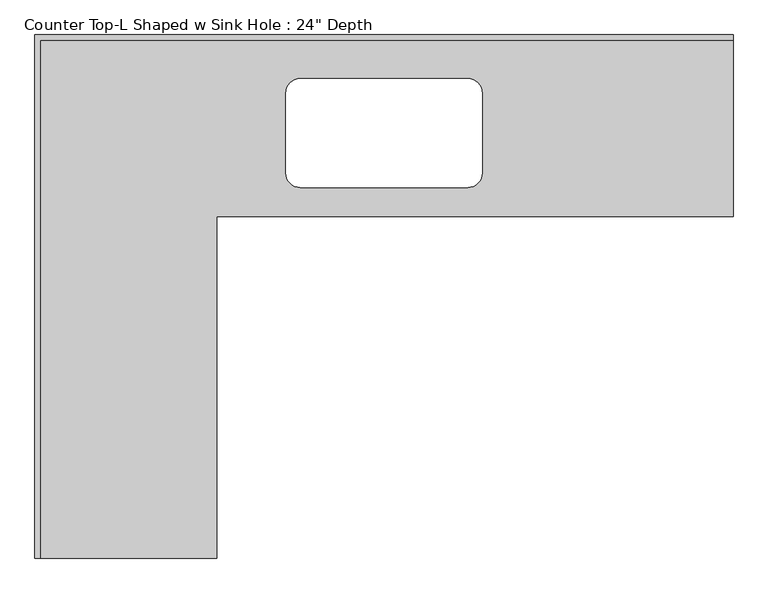
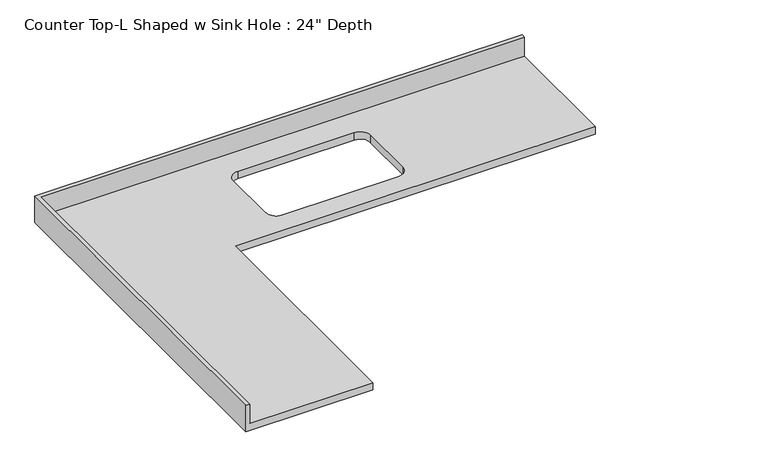
"""IFC4 building model written with IfcOpenShell, lengths in millimetres: furniture geometry."""

from ifc_helpers import new_model, si_unit, frame, origin, place, context, project, spatial, polyline, circle_curve, source, transform, mapped, element, save
from ifc_brep_helpers import plane_surface, revolved_surface, advanced_brep


def furniture_eb5480b5(model_context):
    return source(origin(), model_context, "Body", "AdvancedBrep", [
        advanced_brep(
        [(-565.4622951, -1828.8, 914.4), (-565.4622951, -635.0, 914.4), (1237.9377049, -635.0, 914.4), (1237.9377049, -19.05, 914.4), (-1181.4122951, -19.05, 914.4), (-1181.4122951, -1828.8, 914.4), (310.8377049, -152.4, 914.4), (361.6377049, -203.2, 914.4), (361.6377049, -482.6, 914.4), (310.8377049, -533.4, 914.4), (-273.3622951, -533.4, 914.4), (-324.1622951, -482.6, 914.4), (-324.1622951, -203.2, 914.4), (-273.3622951, -152.4, 914.4), (1237.9377049, 0.0, 876.3), (1237.9377049, -635.0, 876.3), (-565.4622951, -635.0, 876.3), (-565.4622951, -1828.8, 876.3), (-1200.4622951, -1828.8, 876.3), (-1200.4622951, 0.0, 876.3), (310.8377049, -152.4, 876.3), (-273.3622951, -152.4, 876.3), (-324.1622951, -203.2, 876.3), (-324.1622951, -482.6, 876.3), (-273.3622951, -533.4, 876.3), (310.8377049, -533.4, 876.3), (361.6377049, -482.6, 876.3), (361.6377049, -203.2, 876.3), (-1200.4622951, 0.0, 1016.0), (1237.9377049, 0.0, 1016.0), (-1200.4622951, -1828.8, 1016.0), (-1181.4122951, -1828.8, 1016.0), (1237.9377049, -19.05, 1016.0), (-1181.4122951, -19.05, 1016.0)],
        [
            (0, 1),
            (1, 2),
            (2, 3),
            (3, 4),
            (4, 5),
            (5, 0),
            (6, 7, circle_curve(frame((310.8377049, -203.2, 914.4), z_axis=(0.0, 0.0, -1.0), x_axis=(1.0, 0.0, 0.0)), 50.8)),
            (7, 8),
            (8, 9, circle_curve(frame((310.8377049, -482.6, 914.4), z_axis=(0.0, 0.0, -1.0), x_axis=(1.0, 0.0, 0.0)), 50.8)),
            (9, 10),
            (10, 11, circle_curve(frame((-273.3622951, -482.6, 914.4), z_axis=(0.0, 0.0, -1.0), x_axis=(1.0, 0.0, 0.0)), 50.8)),
            (11, 12),
            (12, 13, circle_curve(frame((-273.3622951, -203.2, 914.4), z_axis=(0.0, 0.0, -1.0), x_axis=(1.0, 0.0, 0.0)), 50.8)),
            (13, 6),
            (14, 15),
            (15, 16),
            (16, 17),
            (17, 18),
            (18, 19),
            (19, 14),
            (20, 21),
            (21, 22, circle_curve(frame((-273.3622951, -203.2, 876.3), z_axis=(0.0, 0.0, 1.0), x_axis=(1.0, 0.0, 0.0)), 50.8)),
            (22, 23),
            (23, 24, circle_curve(frame((-273.3622951, -482.6, 876.3), z_axis=(0.0, 0.0, 1.0), x_axis=(1.0, 0.0, 0.0)), 50.8)),
            (24, 25),
            (25, 26, circle_curve(frame((310.8377049, -482.6, 876.3), z_axis=(0.0, 0.0, 1.0), x_axis=(1.0, 0.0, 0.0)), 50.8)),
            (26, 27),
            (27, 20, circle_curve(frame((310.8377049, -203.2, 876.3), z_axis=(0.0, 0.0, 1.0), x_axis=(1.0, 0.0, 0.0)), 50.8)),
            (19, 28),
            (28, 29),
            (29, 14),
            (18, 30),
            (30, 28),
            (17, 0),
            (5, 31),
            (31, 30),
            (16, 1),
            (15, 2),
            (29, 32),
            (32, 3),
            (6, 20),
            (27, 7),
            (26, 8),
            (25, 9),
            (24, 10),
            (23, 11),
            (22, 12),
            (21, 13),
            (31, 33),
            (33, 32),
            (33, 4),
        ],
        [
            plane_surface(frame((-1200.4622951, 0.0, 914.4), z_axis=(0.0, 0.0, 1.0), x_axis=(-1.0, 0.0, 0.0))),
            plane_surface(frame((-1200.4622951, 0.0, 876.3), z_axis=(0.0, 0.0, -1.0), x_axis=(1.0, 0.0, 0.0))),
            plane_surface(frame((1237.9377049, 0.0, 914.4), z_axis=(0.0, 1.0, 0.0), x_axis=(0.0, 0.0, -1.0))),
            plane_surface(frame((-1200.4622951, 0.0, 914.4), z_axis=(-1.0, 0.0, 0.0), x_axis=(0.0, 0.0, -1.0))),
            plane_surface(frame((-1200.4622951, -1828.8, 914.4), z_axis=(0.0, -1.0, 0.0), x_axis=(0.0, 0.0, -1.0))),
            plane_surface(frame((-565.4622951, -1828.8, 914.4), z_axis=(1.0, 0.0, 0.0), x_axis=(0.0, 0.0, -1.0))),
            plane_surface(frame((-565.4622951, -635.0, 914.4), z_axis=(0.0, -1.0, 0.0), x_axis=(0.0, 0.0, -1.0))),
            plane_surface(frame((1237.9377049, -635.0, 914.4), z_axis=(1.0, 0.0, 0.0), x_axis=(0.0, 0.0, -1.0))),
            revolved_surface(polyline([(361.6377049, -203.2, 876.3), (361.6377049, -203.2, 914.4)]), (310.8377049, -203.2, 0.0), (0.0, 0.0, -1.0)),
            plane_surface(frame((361.6377049, -203.2, 914.4), z_axis=(-1.0, 0.0, 0.0), x_axis=(0.0, 0.0, -1.0))),
            revolved_surface(polyline([(361.6377049, -482.6, 876.3), (361.6377049, -482.6, 914.4)]), (310.8377049, -482.6, 0.0), (0.0, 0.0, -1.0)),
            plane_surface(frame((310.8377049, -533.4, 914.4), z_axis=(0.0, 1.0, 0.0), x_axis=(0.0, 0.0, -1.0))),
            revolved_surface(polyline([(-222.56229509999997, -482.6, 876.3), (-222.56229509999997, -482.6, 914.4)]), (-273.3622951, -482.6, 0.0), (0.0, 0.0, -1.0)),
            plane_surface(frame((-324.1622951, -482.6, 914.4), z_axis=(1.0, 0.0, 0.0), x_axis=(0.0, 0.0, -1.0))),
            revolved_surface(polyline([(-222.56229509999997, -203.2, 876.3), (-222.56229509999997, -203.2, 914.4)]), (-273.3622951, -203.2, 0.0), (0.0, 0.0, -1.0)),
            plane_surface(frame((-273.3622951, -152.4, 914.4), z_axis=(0.0, -1.0, 0.0), x_axis=(0.0, 0.0, -1.0))),
            plane_surface(frame((-1200.4622951, 0.0, 1016.0), z_axis=(0.0, 0.0, 1.0), x_axis=(0.0, -1.0, 0.0))),
            plane_surface(frame((-1200.4622951, -19.05, 1016.0), z_axis=(0.0, -1.0, 0.0), x_axis=(0.0, 0.0, -1.0))),
            plane_surface(frame((-1181.4122951, -1828.8, 1016.0), z_axis=(1.0, 0.0, 0.0), x_axis=(0.0, 0.0, -1.0))),
        ],
        [
            (0, [[1, 2, 3, 4, 5, 6], [7, 8, 9, 10, 11, 12, 13, 14]]),
            (1, [[15, 16, 17, 18, 19, 20], [21, 22, 23, 24, 25, 26, 27, 28]]),
            (2, [[-20, 29, 30, 31]]),
            (3, [[-19, 32, 33, -29]]),
            (4, [[-32, -18, 34, -6, 35, 36]]),
            (5, [[-1, -34, -17, 37]]),
            (6, [[-2, -37, -16, 38]]),
            (7, [[-15, -31, 39, 40, -3, -38]]),
            (8, [[-7, 41, -28, 42]]),
            (9, [[-8, -42, -27, 43]]),
            (10, [[-9, -43, -26, 44]]),
            (11, [[-10, -44, -25, 45]]),
            (12, [[-11, -45, -24, 46]]),
            (13, [[-12, -46, -23, 47]]),
            (14, [[-13, -47, -22, 48]]),
            (15, [[-14, -48, -21, -41]]),
            (16, [[-33, -36, 49, 50, -39, -30]]),
            (17, [[-40, -50, 51, -4]]),
            (18, [[-49, -35, -5, -51]]),
        ],
    ),
    ])


if __name__ == "__main__":
    model = new_model("IFC4")
    model_context = context("Model", 3, world=origin())
    ifc_project = project(units=[si_unit("LENGTHUNIT", "METRE", prefix="MILLI")], contexts=[model_context])
    site = spatial("IfcSite", under=ifc_project)
    building = spatial("IfcBuilding", under=site)
    placement = place(None, origin())
    furniture_shape = furniture_eb5480b5(model_context)
    element("IfcFurniture", 1, ObjectType="Counter Top-L Shaped w Sink Hole : 24\" Depth", at=placement, inside=building, context=model_context, shape_type="MappedRepresentation", body=[
        mapped(furniture_shape, transform((0.0, 0.0, 0.0), x_axis=(1.0, 0.0, 0.0), y_axis=(0.0, 1.0, 0.0), z_axis=(0.0, 0.0, 1.0))),
    ])
    save(model, "model.ifc")

# Revit data of these elements
# Type "Counter Top-L Shaped w Sink Hole : 24\" Depth"
#   Assembly Code = "C1030400"
#   Counter Thickness = 0' - 1 1/2"
#   Depth = 2' - 1"
#   Height = 3' - 0"
#   Length - Leg 1 [instance default] = 8' - 0"
#   Length - Leg 2 [instance default] = 6' - 0"
#   Sink Location [instance default] = 2' - 10 1/2"
#   Sink Location To Wall [instance default] = 0' - 6"
#   Sink Opening Depth [instance default] = 1' - 3"
#   Sink Opening Width [instance default] = 2' - 3"
#   Counter Top Material = none
#   Default Elevation = 0
# Element 1 (IfcFurniture, "Counter Top-L Shaped w Sink Hole : 24\" Depth")
#   Materials on its faces: "Counter Top"
# Materials
#   "Counter Top": class "Wood", colour RGB 226 177 128, transparency 0
